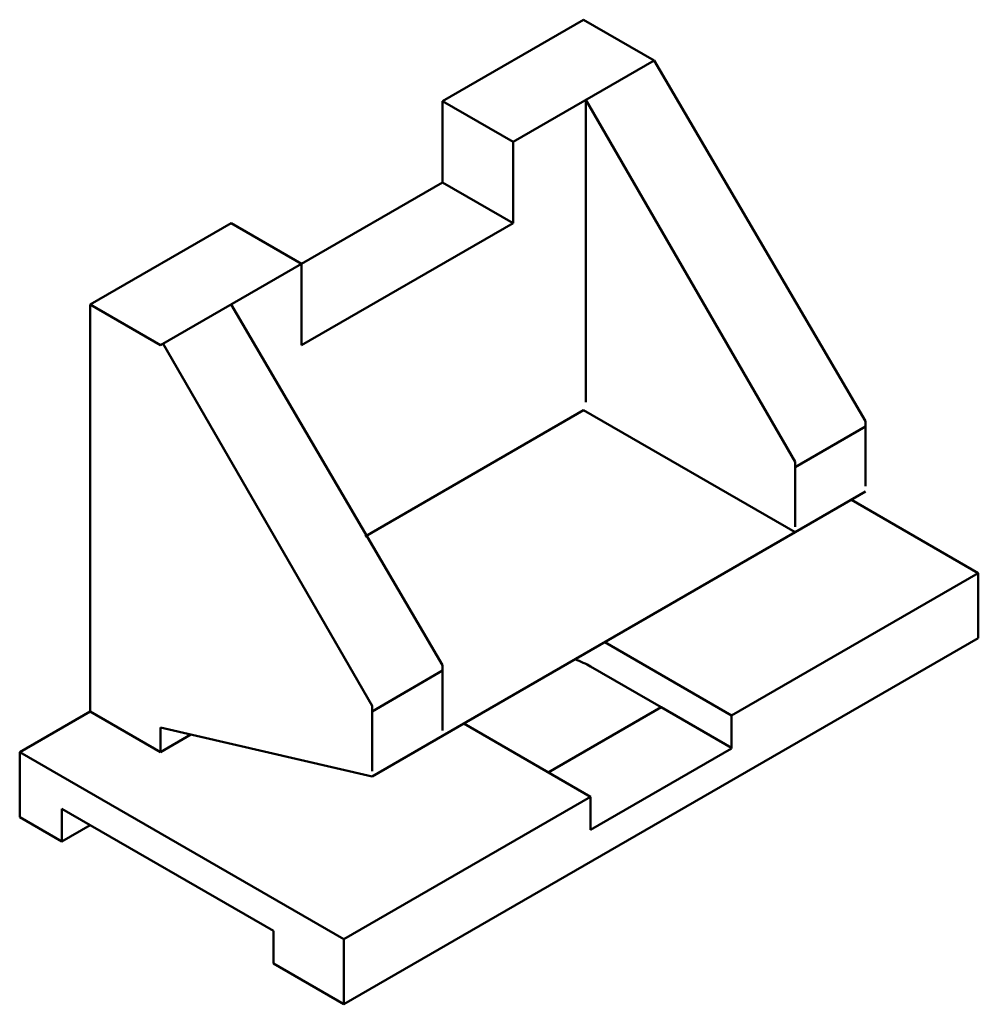
# Model space of a CAD drawing. Units: millimetres. Extents: x 2608 to 5381, y 822 to 1708.
# Tile 1 of 1: x 2608.1 to 2725.9, y 822 to 943. Entities that reach past the tile are written whole.
import ezdxf

# ---------------------------------------------------------------- set-up
doc = ezdxf.new("R2010")
doc.units = ezdxf.units.MM
doc.layers.add('M-OUTL', color=7, linetype='Continuous', lineweight=50)

msp = doc.modelspace()

# ---------------------------------------------------------------- linework, layer by layer
at = {"layer": 'M-OUTL'}
for p, q in [((2660.1, 932.98), (2677.42, 942.98)), ((2686.09, 937.98), (2677.42, 942.98)), ((2668.76, 927.98), (2686.09, 937.98)), ((2686.09, 937.98), (2712.07, 893.64)), ((2660.1, 932.98), (2668.76, 927.98)), ((2660.1, 932.98), (2660.1, 922.98)), ((2703.41, 888.64), (2677.71, 933.14)), ((2677.71, 933.14), (2677.71, 895.99)), ((2668.76, 917.98), (2668.76, 927.98)), ((2642.78, 912.98), (2660.1, 922.98)), ((2660.1, 922.98), (2668.76, 917.98)), ((2616.8, 907.98), (2634.12, 917.98)), ((2642.78, 912.98), (2634.12, 917.98)), ((2668.76, 917.98), (2642.78, 902.98)), ((2625.46, 902.98), (2642.78, 912.98)), ((2642.78, 912.98), (2642.78, 902.98)), ((2616.8, 857.98), (2616.8, 907.98)), ((2616.8, 907.98), (2625.46, 902.98)), ((2634.12, 907.98), (2660.1, 863.64)), ((2651.44, 858.64), (2625.75, 903.14)), ((2650.58, 879.48), (2677.42, 894.98)), ((2677.42, 894.98), (2703.41, 879.98)), ((2712.07, 893.64), (2712.07, 888.64)), ((2703.41, 887.98), (2712.07, 892.98)), ((2703.41, 880.64), (2703.41, 888.64)), ((2712.07, 888.64), (2712.07, 885.64)), ((2703.41, 879.98), (2712.07, 884.98)), ((2725.92, 874.98), (2710.33, 883.98)), ((2660.1, 854.98), (2703.41, 879.98)), ((2695.61, 857.48), (2725.92, 874.98)), ((2725.92, 871.98), (2725.92, 874.98)), ((2725.92, 866.98), (2725.92, 871.98)), ((2647.98, 821.98), (2725.92, 866.98)), ((2695.61, 857.48), (2680.02, 866.48)), ((2651.44, 857.98), (2660.1, 862.98)), ((2660.1, 863.64), (2660.1, 858.64)), ((2686.95, 858.48), (2678.29, 863.48)), ((2608.14, 852.98), (2616.8, 857.98)), ((2625.46, 852.98), (2616.8, 857.98)), ((2651.44, 850.64), (2651.44, 858.64)), ((2660.1, 858.64), (2660.1, 855.64)), ((2673.09, 850.48), (2686.95, 858.48)), ((2695.61, 853.48), (2686.95, 858.48)), ((2695.61, 857.48), (2695.61, 853.41)), ((2651.44, 849.98), (2625.46, 855.98)), ((2625.46, 855.98), (2625.46, 852.98)), ((2678.29, 847.48), (2662.7, 856.48)), ((2629.17, 855.12), (2625.46, 852.98)), ((2651.44, 849.98), (2660.1, 854.98)), ((2695.61, 853.41), (2678.29, 843.41)), ((2647.98, 829.98), (2608.14, 852.98)), ((2608.14, 852.98), (2608.14, 852.98)), ((2608.14, 844.98), (2608.14, 852.98)), ((2647.98, 829.98), (2678.29, 847.48)), ((2678.29, 843.41), (2678.29, 847.48)), ((2639.32, 831), (2613.34, 846)), ((2613.34, 841.98), (2613.34, 845.98)), ((2613.34, 841.98), (2608.14, 844.98)), ((2613.34, 841.98), (2616.8, 843.98)), ((2639.32, 826.98), (2639.32, 831)), ((2647.98, 827.98), (2647.98, 829.98)), ((2647.98, 821.98), (2647.98, 827.98)), ((2647.98, 821.98), (2639.32, 826.98))]:
    msp.add_line(p, q, dxfattribs=at)
msp.add_ellipse((2669.63, 858.48), major_axis=(12.25, 0), ratio=0.57735, start_param=0.785398, end_param=0.986756, dxfattribs=at)

doc.saveas('drawing.dxf')
